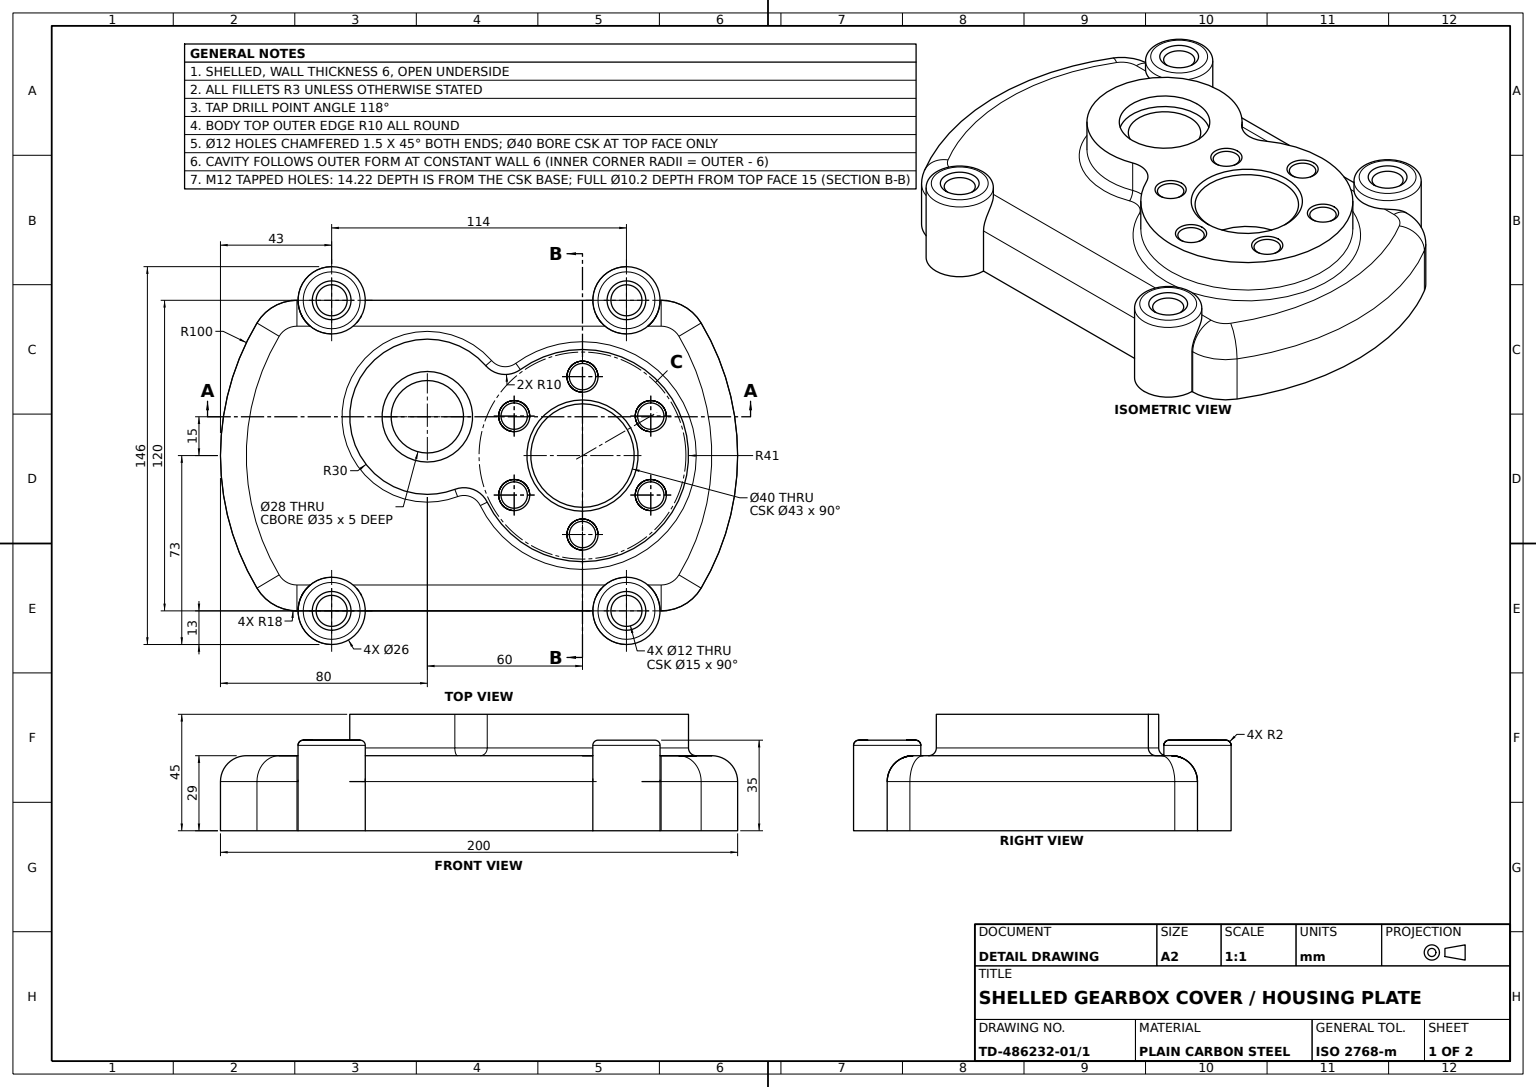
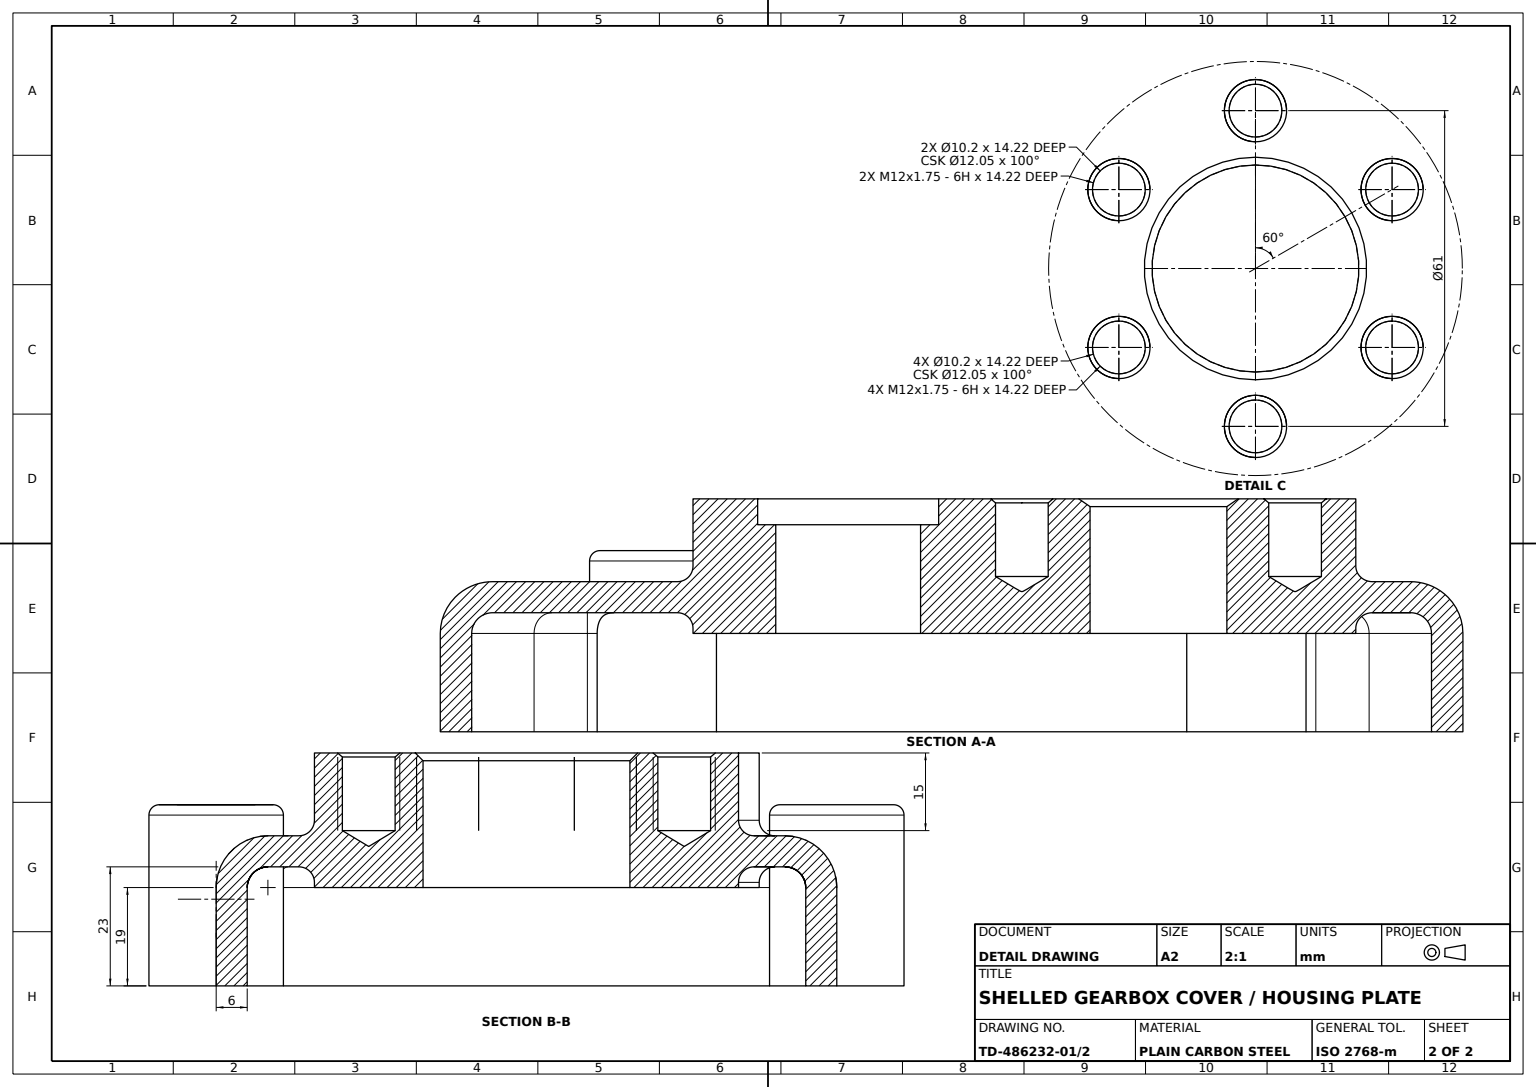
from build123d import *

# Parameters (mm, degrees)
HOUSING_BASE_DEPTH                          = 29
BASE_CORNER_FILLET_R18_R                    = 18
BASE_EDGE_FILLET_R10_R                      = 10
HOUSING_SHELL_6MM_T                         = -6
BEARING_START                               = 45
BEARING_BOSS_DEPTH                          = 26
SKETCH2_9_R                                 = 20
SKETCH2_9_R_2                               = 14
BEARING_BORES_DEPTH                         = 126.00000008
BOSS_START                                  = 45
SKETCH2_10_R                                = 17.5
BOSS_RECESS_CUT_5MM_DEPTH                   = 5
BOSS_ROOT_FILLET_R3_R                       = 3
BOSS_SHELL_FILLET_R3_R                      = 3
BEARING_BORE_CHAMFER_1_5X45_SIZE            = 1.5
SKETCH2_11_R                                = 13
MOUNTING_LUGS_DEPTH                         = 35
SKETCH2_12_R                                = 6
LUG_HOLES_DEPTH                             = 35
LUG_HOLE_MIRROR_AT_THE_SECOND_PLANE_COPY_R  = 6
LUG_HOLE_MIRROR_AT_THE_SECOND_PLANE_2_DEPTH = 35
LUG_HOLE_CHAMFER_1_5X45_SIZE                = 1.5
LUG_FILLET_R2_R                             = 2
TAPPED_HOLE_PATTERN_6X_COUNT                = 6


with BuildPart() as part:
    # Housing Master Sketch → Housing Base (new body)
    with BuildSketch(Plane(origin=(0, 0, 0), x_dir=(1, 0, 0), z_dir=(0, 1, 0))):
        with BuildLine():
            Line((-80, 60), (80, 60))
            ThreePointArc((80, 60), (100, 0), (80, -60))
            Line((80, -60), (-80, -60))
            ThreePointArc((-80, -60), (-100, 0), (-80, 60))
        make_face()
    extrude(amount=HOUSING_BASE_DEPTH)

    # Base Corner Fillet R18
    base_corner_fillet_r18_edges = [part.edges().sort_by_distance(p)[0] for p in [
        (-80, 14.5, -60),
        (80, 14.5, -60),
        (80, 14.5, 60),
        (-80, 14.5, 60),
    ]]
    fillet(base_corner_fillet_r18_edges, radius=BASE_CORNER_FILLET_R18_R)

    # Base Edge Fillet R10
    base_edge_fillet_r10_edges = [part.edges().sort_by_distance(p)[0] for p in [
        (0, 29, 60),
        (-100, 29, 0),
        (100, 29, 0),
        (0, 29, -60),
        (-79.316833816, 29, -57.651696705),
        (79.316833816, 29, -57.651696705),
        (79.316833816, 29, 57.651696705),
        (-79.316833816, 29, 57.651696705),
    ]]
    fillet(base_edge_fillet_r10_edges, radius=BASE_EDGE_FILLET_R10_R)

    # Housing Shell 6mm
    housing_shell_6mm_openings = [part.faces().sort_by_distance(p)[0] for p in [
        (0, 0, 0),
    ]]
    offset(amount=HOUSING_SHELL_6MM_T, openings=housing_shell_6mm_openings, kind=Kind.INTERSECTION)

    # Sketch2_7 → Bearing Boss (add)
    with BuildSketch(Plane(origin=(0, 0, 0), x_dir=(1, 0, 0), z_dir=(0, 1, 0)).offset(BEARING_START)):
        with BuildLine():
            ThreePointArc((3.166776615, -18.008710533), (79.775842506, -9.943960626), (15.974784323, 33.223320299))
            ThreePointArc((15.974784323, 33.223320299), (8.985746764, 31.390531603), (2.586231716, 34.744926864))
            ThreePointArc((2.586231716, 34.744926864), (-49.104275004, 22.276068751), (-9.362702304, -13.050809217))
            ThreePointArc((-9.362702304, -13.050809217), (-2.137532433, -13.102585185), (3.166776615, -18.008710533))
        make_face()
    extrude(amount=-BEARING_BOSS_DEPTH)

    # Sketch2_9 → Bearing Bores (cut, through all)
    with BuildSketch(Plane(origin=(0, 0, 0), x_dir=(1, 0, 0), z_dir=(0, 1, 0))):
        with Locations(Location((40, 0, 0), (0, 0, 90))):
            Circle(SKETCH2_9_R)
        with Locations(Location((-20, 15, 0), (0, 0, 90))):
            Circle(SKETCH2_9_R_2)
    extrude(amount=BEARING_BORES_DEPTH, mode=Mode.SUBTRACT)

    # Sketch2_10 → Boss Recess Cut 5mm (cut)
    with BuildSketch(Plane(origin=(0, 0, 0), x_dir=(1, 0, 0), z_dir=(0, 1, 0)).offset(BOSS_START)):
        with Locations(Location((-20, 15, 0), (0, 0, 270))):
            Circle(SKETCH2_10_R)
    extrude(amount=-BOSS_RECESS_CUT_5MM_DEPTH, mode=Mode.SUBTRACT)

    # Boss Root Fillet R3
    boss_root_fillet_r3_edges = [part.edges().sort_by_distance(p)[0] for p in [
        (8.985746764, 29, -31.390531603),
        (-2.137532433, 29, 13.102585185),
        (79.775842506, 29, 9.943960626),
        (-49.104275004, 29, -22.276068751),
    ]]
    fillet(boss_root_fillet_r3_edges, radius=BOSS_ROOT_FILLET_R3_R)

    # Boss Shell Fillet R3
    boss_shell_fillet_r3_edges = [part.edges().sort_by_distance(p)[0] for p in [
        (-49.104275004, 23, -22.276068751),
        (-2.137532433, 23, 13.102585185),
        (79.775842506, 23, 9.943960626),
        (8.985746764, 23, -31.390531603),
    ]]
    fillet(boss_shell_fillet_r3_edges, radius=BOSS_SHELL_FILLET_R3_R)

    # Bearing Bore Chamfer 1.5x45
    bearing_bore_chamfer_1_5x45_edges = [part.edges().sort_by_distance(p)[0] for p in [
        (40, 45, 20),
    ]]
    chamfer(bearing_bore_chamfer_1_5x45_edges, length=BEARING_BORE_CHAMFER_1_5X45_SIZE)

    # Sketch2_11 → Mounting Lugs (add)
    with BuildSketch(Plane(origin=(0, 0, 0), x_dir=(1, 0, 0), z_dir=(0, 1, 0))):
        with Locations(Location((-57, 60, 0), (0, 0, 180))):
            Circle(SKETCH2_11_R)
        with Locations(Location((57, 60, 0), (0, 0, 90))):
            Circle(SKETCH2_11_R)
        with Locations(Location((57, -60, 0), (0, 0, 50.284862768))):
            Circle(SKETCH2_11_R)
        with Locations(Location((-57, -60, 0), (0, 0, 90))):
            Circle(SKETCH2_11_R)
    extrude(amount=MOUNTING_LUGS_DEPTH)

    # Sketch2_12 → Lug Holes (cut)
    with BuildSketch(Plane(origin=(0, 0, 0), x_dir=(1, 0, 0), z_dir=(0, 1, 0))):
        with Locations(Location((-57, 60, 0), (0, 0, 270))):
            Circle(SKETCH2_12_R)
    lug_holes = extrude(amount=LUG_HOLES_DEPTH, mode=Mode.SUBTRACT)

    # Lug Hole Mirror: Lug Holes across plane
    add(lug_holes.mirror(Plane(origin=(0, 0, 0), x_dir=(0, 0, 1), z_dir=(1, 0, 0))), mode=Mode.SUBTRACT)

    # Lug Hole Mirror at the second plane: Lug Holes across plane
    add(lug_holes.mirror(Plane.XY), mode=Mode.SUBTRACT)

    # Lug Hole Mirror at the second plane copy → Lug Hole Mirror at the second plane  2 (cut)
    with BuildSketch(Plane(origin=(0, 0, 0), x_dir=(-1, 0, 0), z_dir=(0, 1, 0))):
        with Locations(Location((-57, 60, 0), (0, 0, 270))):
            Circle(LUG_HOLE_MIRROR_AT_THE_SECOND_PLANE_COPY_R)
    extrude(amount=LUG_HOLE_MIRROR_AT_THE_SECOND_PLANE_2_DEPTH, mode=Mode.SUBTRACT)

    # Lug Hole Chamfer 1.5x45
    lug_hole_chamfer_1_5x45_edges = [part.edges().sort_by_distance(p)[0] for p in [
        (-57, 35, -66),
        (-57, 35, 66),
        (57, 35, -66),
        (57, 0, -66),
        (57, 35, 66),
    ]]
    chamfer(lug_hole_chamfer_1_5x45_edges, length=LUG_HOLE_CHAMFER_1_5X45_SIZE)

    # Lug Fillet R2
    lug_fillet_r2_edges = [part.edges().sort_by_distance(p)[0] for p in [
        (-57, 35, 73),
        (48.693376137, 35, 70),
        (57, 35, -47),
        (-44, 35, -60),
    ]]
    fillet(lug_fillet_r2_edges, radius=LUG_FILLET_R2_R)

    # Sketch31 → Cover Tapped Hole M12 (revolve, cut)
    with BuildSketch(Plane(origin=(40, 45, -30.5), x_dir=(0, 0, 1), z_dir=(1, 0, 0))):
        Polygon((0, 0), (0, 18.064389157), (5.1, 15), (5.1, 0.776167159), (6.025, 0), align=None)
    cover_tapped_hole_m12 = revolve(axis=Axis((40, 51.35, -30.5), (0, -1, 0)), mode=Mode.SUBTRACT)

    # Tapped Hole Pattern 6x: Cover Tapped Hole M12 ×6 about axis
    tapped_hole_pattern_6x_axis = Axis((40, 0, 0), (0, 1, 0))
    for i in range(1, TAPPED_HOLE_PATTERN_6X_COUNT):
        add(cover_tapped_hole_m12.rotate(tapped_hole_pattern_6x_axis, i * 360 / TAPPED_HOLE_PATTERN_6X_COUNT), mode=Mode.SUBTRACT)


solid = part.part
